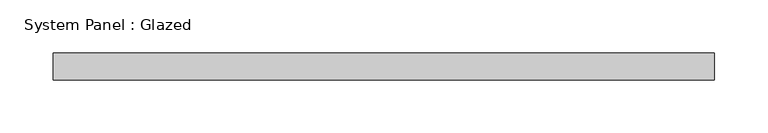
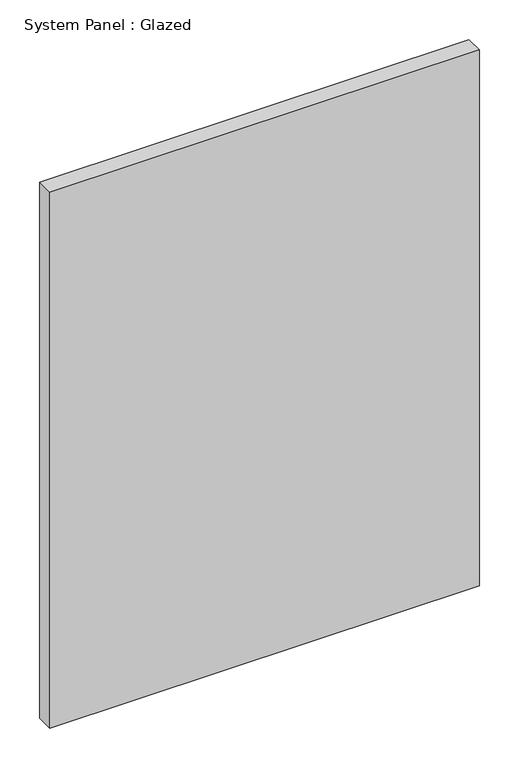
"""IFC4 building model written with IfcOpenShell, lengths in millimetres: plate geometry, System Panel : Glazed."""

from ifc_helpers import new_model, si_unit, origin, origin_with_axes, place, context, project, spatial, polyline, outline, extrude, source, transform, mapped, element, save


def system_panel_glazed_1601ec89(model_context):
    return source(origin(), model_context, "Body", "SweptSolid", [
        extrude(outline(polyline([(311.15, 19.05), (-311.15, 19.05), (-311.15, 44.45), (311.15, 44.45), (311.15, 19.05)])), origin_with_axes(), (0.0, 0.0, 1.0), 820.9261324),
    ])


if __name__ == "__main__":
    model = new_model("IFC4")
    model_context = context("Model", 3, world=origin())
    ifc_project = project(units=[si_unit("LENGTHUNIT", "METRE", prefix="MILLI")], contexts=[model_context])
    site = spatial("IfcSite", under=ifc_project)
    building = spatial("IfcBuilding", under=site)
    placement = place(None, origin())
    system_panel_glazed_shape = system_panel_glazed_1601ec89(model_context)
    element("IfcPlate", 1, ObjectType="System Panel : Glazed", at=placement, inside=building, context=model_context, shape_type="MappedRepresentation", body=[
        mapped(system_panel_glazed_shape, transform((0.0, 0.0, 0.0), x_axis=(1.0, 0.0, 0.0), y_axis=(0.0, 1.0, 0.0), z_axis=(0.0, 0.0, 1.0))),
    ])
    save(model, "model.ifc")

# Revit data of these elements
# Type "System Panel : Glazed"
#   Construction Type Id = "GSP4R"
#   Analytic Construction = "1/8 in Pilkington single glazing"
#   Visual Light Transmittance = 0.9
#   Solar Heat Gain Coefficient = 0.86
#   Heat Transfer Coefficient (U) = 1.18115 BTU/(h·ft²·°F)
#   Define Thermal Properties by = 1
# Element 1 (IfcPlate, "System Panel : Glazed")
#   Materials on its faces: "Glass"
# Materials
#   "Glass": class "Glass", colour RGB 0 128 192, transparency 0.75, Description = "Soda Lime Glass", Cost = 0
